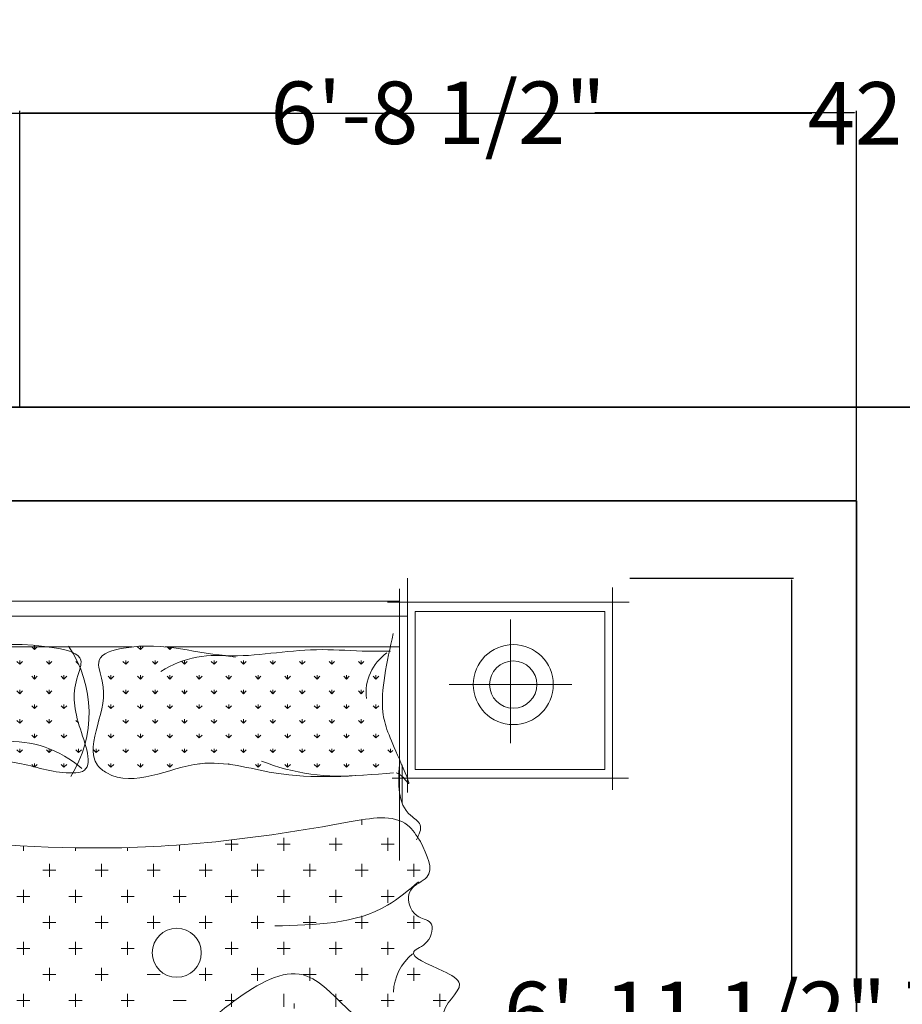
# Model space of a CAD drawing. Units: inches. Extents: x -26 to 575, y -18 to 513.
# Tile 14 of 28: x 189 to 274, y 418 to 513. Entities that reach past the tile are written whole.
import ezdxf

# ---------------------------------------------------------------- set-up
doc = ezdxf.new("R2010")
doc.units = ezdxf.units.IN
doc.header["$MEASUREMENT"] = 0
for name, color, linetype, lineweight in [('A-ANNO-DIMS', 2, 'Continuous', 18), ('A-WALL', 7, 'Continuous', 35), ('Furniture', 8, 'Continuous', 15)]:
    doc.layers.add(name, color=color, linetype=linetype, lineweight=lineweight)
doc.styles.get("Standard").update_dxf_attribs({"font": 'arial.ttf', "height": 6})
doc.dimstyles.get("Standard").update_dxf_attribs({"dimtxt": 6, "dimasz": 0.18, "dimexe": 0.18, "dimexo": 0.0625, "dimgap": 0.09, "dimtad": 0, "dimtih": 1, "dimtoh": 1, "dimzin": 0, "dimdsep": 46, "dimlunit": 3, "dimtxsty": 'Standard', "dimcen": 0.09, "dimadec": 0, "dimazin": 0, "dimtfac": 1, "dimtofl": 0, "dimtmove": 0, "dimatfit": 3, "dimfxl": 1, "dimtolj": 1, "dimtzin": 0, "dimarcsym": 0})

# ---------------------------------------------------------------- blocks, each defined once
blk = doc.blocks.new('*D1')
at = {"layer": 'A-ANNO-DIMS', "color": 0, "lineweight": -2, "transparency": 16777216}
for p, q in [((18.177, 475.57), (18.177, 503.937)), ((18.357, 503.757), (264.875, 503.757)), ((521.997, 503.757), (275.479, 503.757)), ((522.177, 475.57), (522.177, 503.937))]:
    blk.add_line(p, q, dxfattribs=at)
at = {"layer": 'A-ANNO-DIMS', "color": 0, "transparency": 16777216}
for points in [[(18.357, 503.787), (18.357, 503.727), (18.177, 503.757)], [(521.997, 503.787), (521.997, 503.727), (522.177, 503.757)]]:
    blk.add_solid(points, dxfattribs=at)
at = {"layer": 'Defpoints', "color": 0, "transparency": 16777216}
for p in [(522.177, 503.757), (18.177, 475.508), (522.177, 475.508)]:
    blk.add_point(p, dxfattribs=at)
at = {"layer": 'A-ANNO-DIMS', "color": 0, "transparency": 16777216, "insert": (270.177, 503.757), "char_height": 6, "attachment_point": 5}
blk.add_mtext("\\A1;42'", dxfattribs=at)
blk = doc.blocks.new('BED-DOUBLE-WITH-NIGHTSTANDS')
for p, q in [((82.669, 83.361), (82.669, 62.761)), ((81.883, 82.344), (81.883, 56.232)), ((102.354, 63.031), (102.354, 82.461)), ((21.24, 81.17), (81.883, 81.17)), ((103.97, 81.078), (80.744, 81.078)), ((82.669, 79.717), (21.062, 79.717)), ((101.633, 80.153), (83.411, 80.153)), ((83.411, 80.153), (83.411, 64.968)), ((101.633, 64.968), (101.633, 80.153)), ((92.567, 79.403), (92.567, 67.508)), ((56.226, 76.764), (41.357, 76.764)), ((46.825, 76.507), (46.56, 76.772)), ((46.825, 76.507), (47.09, 76.772)), ((46.826, 76.507), (46.826, 76.882)), ((57.003, 76.507), (56.737, 76.772)), ((57.003, 76.507), (57.003, 76.828)), ((57.003, 76.507), (57.268, 76.772)), ((81.883, 76.764), (59.394, 76.764)), ((59.831, 76.507), (59.594, 76.744)), ((59.831, 76.507), (59.831, 76.717)), ((59.831, 76.507), (60.018, 76.694)), ((45.411, 75.093), (45.146, 75.358)), ((45.411, 75.093), (45.411, 75.468)), ((45.411, 75.093), (45.676, 75.358)), ((48.239, 75.093), (47.974, 75.358)), ((48.239, 75.093), (48.505, 75.358)), ((48.24, 75.093), (48.24, 75.468)), ((51.068, 75.093), (50.803, 75.358)), ((51.068, 75.093), (51.068, 75.099)), ((51.068, 75.093), (51.07, 75.095)), ((53.004, 75.337), (53.025, 75.358)), ((55.588, 75.093), (55.323, 75.358)), ((55.588, 75.093), (55.854, 75.358)), ((55.589, 75.093), (55.589, 75.468)), ((58.417, 75.093), (58.152, 75.358)), ((58.417, 75.093), (58.417, 75.468)), ((58.417, 75.093), (58.682, 75.358)), ((61.245, 75.093), (60.98, 75.358)), ((61.245, 75.093), (61.51, 75.358)), ((61.246, 75.093), (61.246, 75.468)), ((64.074, 75.093), (63.809, 75.358)), ((64.074, 75.093), (64.074, 75.468)), ((64.074, 75.093), (64.339, 75.358)), ((66.902, 75.093), (66.637, 75.358)), ((66.902, 75.093), (67.167, 75.358)), ((66.903, 75.093), (66.903, 75.468)), ((69.731, 75.093), (69.465, 75.358)), ((69.731, 75.093), (69.731, 75.468)), ((69.731, 75.093), (69.996, 75.358)), ((72.559, 75.093), (72.294, 75.358)), ((72.559, 75.093), (72.559, 75.468)), ((72.559, 75.093), (72.824, 75.358)), ((75.387, 75.093), (75.122, 75.358)), ((75.387, 75.093), (75.653, 75.358)), ((75.388, 75.093), (75.388, 75.468)), ((78.216, 75.093), (77.951, 75.358)), ((78.216, 75.093), (78.216, 75.468)), ((78.216, 75.093), (78.481, 75.358)), ((46.825, 73.679), (46.56, 73.944)), ((46.825, 73.679), (47.09, 73.944)), ((46.826, 73.678), (46.826, 74.053)), ((49.654, 73.679), (49.388, 73.944)), ((49.654, 73.678), (49.654, 74.053)), ((49.654, 73.679), (49.919, 73.944)), ((54.174, 73.679), (53.909, 73.944)), ((54.174, 73.679), (54.439, 73.944)), ((54.175, 73.678), (54.175, 74.053)), ((57.003, 73.679), (56.737, 73.944)), ((57.003, 73.678), (57.003, 74.053)), ((57.003, 73.679), (57.268, 73.944)), ((59.831, 73.679), (59.566, 73.944)), ((59.831, 73.678), (59.831, 74.053)), ((59.831, 73.679), (60.096, 73.944)), ((62.66, 73.679), (62.394, 73.944)), ((62.66, 73.678), (62.66, 74.053)), ((62.66, 73.679), (62.925, 73.944)), ((65.488, 73.679), (65.223, 73.944)), ((65.488, 73.678), (65.488, 74.053)), ((65.488, 73.679), (65.753, 73.944)), ((68.316, 73.679), (68.051, 73.944)), ((68.316, 73.679), (68.582, 73.944)), ((68.317, 73.678), (68.317, 74.053)), ((71.145, 73.679), (70.88, 73.944)), ((71.145, 73.678), (71.145, 74.053)), ((71.145, 73.679), (71.41, 73.944)), ((73.973, 73.679), (73.708, 73.944)), ((73.973, 73.679), (74.238, 73.944)), ((73.974, 73.678), (73.974, 74.053)), ((76.802, 73.679), (76.536, 73.944)), ((76.802, 73.678), (76.802, 74.053)), ((76.802, 73.679), (77.067, 73.944)), ((79.63, 73.679), (79.365, 73.944)), ((79.63, 73.678), (79.63, 74.053)), ((79.63, 73.679), (79.895, 73.944)), ((98.466, 73.144), (86.668, 73.144)), ((45.411, 72.265), (45.146, 72.53)), ((45.411, 72.264), (45.411, 72.639)), ((45.411, 72.265), (45.676, 72.53)), ((48.239, 72.265), (47.974, 72.53)), ((48.239, 72.265), (48.505, 72.53)), ((48.24, 72.264), (48.24, 72.639)), ((55.588, 72.265), (55.323, 72.53)), ((55.588, 72.265), (55.854, 72.53)), ((55.589, 72.264), (55.589, 72.639)), ((58.417, 72.265), (58.152, 72.53)), ((58.417, 72.264), (58.417, 72.639)), ((58.417, 72.265), (58.682, 72.53)), ((61.245, 72.265), (60.98, 72.53)), ((61.245, 72.265), (61.51, 72.53)), ((61.246, 72.264), (61.246, 72.639)), ((64.074, 72.265), (63.809, 72.53)), ((64.074, 72.264), (64.074, 72.639)), ((64.074, 72.265), (64.339, 72.53)), ((66.902, 72.265), (66.637, 72.53)), ((66.902, 72.265), (67.167, 72.53)), ((66.903, 72.264), (66.903, 72.639)), ((69.731, 72.265), (69.465, 72.53)), ((69.731, 72.264), (69.731, 72.639)), ((69.731, 72.265), (69.996, 72.53)), ((72.559, 72.265), (72.294, 72.53)), ((72.559, 72.264), (72.559, 72.639)), ((72.559, 72.265), (72.824, 72.53)), ((75.387, 72.265), (75.122, 72.53)), ((75.387, 72.265), (75.653, 72.53)), ((75.388, 72.264), (75.388, 72.639)), ((78.216, 72.265), (77.951, 72.53)), ((78.216, 72.264), (78.216, 72.639)), ((78.216, 72.265), (78.481, 72.53)), ((46.825, 70.85), (46.56, 71.116)), ((46.825, 70.85), (47.09, 71.116)), ((46.826, 70.85), (46.826, 71.225)), ((49.654, 70.85), (49.388, 71.116)), ((49.654, 70.85), (49.654, 71.225)), ((49.654, 70.85), (49.919, 71.116)), ((54.174, 70.85), (53.909, 71.116)), ((54.174, 70.85), (54.439, 71.116)), ((54.175, 70.85), (54.175, 71.225)), ((57.003, 70.85), (56.737, 71.116)), ((57.003, 70.85), (57.003, 71.225)), ((57.003, 70.85), (57.268, 71.116)), ((59.831, 70.85), (59.566, 71.116)), ((59.831, 70.85), (59.831, 71.225)), ((59.831, 70.85), (60.096, 71.116)), ((62.66, 70.85), (62.394, 71.116)), ((62.66, 70.85), (62.66, 71.225)), ((62.66, 70.85), (62.925, 71.116)), ((65.488, 70.85), (65.223, 71.116)), ((65.488, 70.85), (65.488, 71.225)), ((65.488, 70.85), (65.753, 71.116)), ((68.316, 70.85), (68.051, 71.116)), ((68.316, 70.85), (68.582, 71.116)), ((68.317, 70.85), (68.317, 71.225)), ((71.145, 70.85), (70.88, 71.116)), ((71.145, 70.85), (71.145, 71.225)), ((71.145, 70.85), (71.41, 71.116)), ((73.973, 70.85), (73.708, 71.116)), ((73.973, 70.85), (74.238, 71.116)), ((73.974, 70.85), (73.974, 71.225)), ((76.802, 70.85), (76.536, 71.116)), ((76.802, 70.85), (76.802, 71.225)), ((76.802, 70.85), (77.067, 71.116)), ((79.63, 70.85), (79.365, 71.116)), ((79.63, 70.85), (79.63, 71.225)), ((79.63, 70.85), (79.895, 71.116)), ((45.411, 69.436), (45.146, 69.701)), ((45.411, 69.436), (45.411, 69.811)), ((45.411, 69.436), (45.676, 69.701)), ((48.239, 69.436), (47.974, 69.701)), ((48.239, 69.436), (48.505, 69.701)), ((48.24, 69.436), (48.24, 69.811)), ((51.052, 69.452), (50.803, 69.701)), ((53.007, 69.683), (53.025, 69.701)), ((55.588, 69.436), (55.323, 69.701)), ((55.588, 69.436), (55.854, 69.701)), ((55.589, 69.436), (55.589, 69.811)), ((58.417, 69.436), (58.152, 69.701)), ((58.417, 69.436), (58.417, 69.811)), ((58.417, 69.436), (58.682, 69.701)), ((61.245, 69.436), (60.98, 69.701)), ((61.245, 69.436), (61.51, 69.701)), ((61.246, 69.436), (61.246, 69.811)), ((64.074, 69.436), (63.809, 69.701)), ((64.074, 69.436), (64.074, 69.811)), ((64.074, 69.436), (64.339, 69.701)), ((66.902, 69.436), (66.637, 69.701)), ((66.902, 69.436), (67.167, 69.701)), ((66.903, 69.436), (66.903, 69.811)), ((69.731, 69.436), (69.465, 69.701)), ((69.731, 69.436), (69.731, 69.811)), ((69.731, 69.436), (69.996, 69.701)), ((72.559, 69.436), (72.294, 69.701)), ((72.559, 69.436), (72.559, 69.811)), ((72.559, 69.436), (72.824, 69.701)), ((75.387, 69.436), (75.122, 69.701)), ((75.387, 69.436), (75.653, 69.701)), ((75.388, 69.436), (75.388, 69.811)), ((78.216, 69.436), (77.951, 69.701)), ((78.216, 69.436), (78.216, 69.811)), ((78.216, 69.436), (78.481, 69.701)), ((46.825, 68.022), (46.56, 68.287)), ((46.825, 68.022), (47.09, 68.287)), ((46.826, 68.022), (46.826, 68.397)), ((49.654, 68.022), (49.388, 68.287)), ((49.654, 68.022), (49.654, 68.397)), ((49.654, 68.022), (49.919, 68.287)), ((54.174, 68.022), (53.909, 68.287)), ((54.174, 68.022), (54.439, 68.287)), ((54.175, 68.022), (54.175, 68.397)), ((57.003, 68.022), (56.737, 68.287)), ((57.003, 68.022), (57.003, 68.397)), ((57.003, 68.022), (57.268, 68.287)), ((59.831, 68.022), (59.566, 68.287)), ((59.831, 68.022), (59.831, 68.397)), ((59.831, 68.022), (60.096, 68.287)), ((62.66, 68.022), (62.394, 68.287)), ((62.66, 68.022), (62.66, 68.397)), ((62.66, 68.022), (62.925, 68.287)), ((65.488, 68.022), (65.223, 68.287)), ((65.488, 68.022), (65.488, 68.397)), ((65.488, 68.022), (65.753, 68.287)), ((68.316, 68.022), (68.051, 68.287)), ((68.316, 68.022), (68.582, 68.287)), ((68.317, 68.022), (68.317, 68.397)), ((71.145, 68.022), (70.88, 68.287)), ((71.145, 68.022), (71.145, 68.397)), ((71.145, 68.022), (71.41, 68.287)), ((73.973, 68.022), (73.708, 68.287)), ((73.973, 68.022), (74.238, 68.287)), ((73.974, 68.022), (73.974, 68.397)), ((76.802, 68.022), (76.536, 68.287)), ((76.802, 68.022), (76.802, 68.397)), ((76.802, 68.022), (77.067, 68.287)), ((79.63, 68.022), (79.365, 68.287)), ((79.63, 68.022), (79.63, 68.397)), ((79.63, 68.022), (79.895, 68.287)), ((45.411, 66.608), (45.146, 66.873)), ((45.411, 66.607), (45.411, 66.982)), ((45.411, 66.608), (45.676, 66.873)), ((48.239, 66.608), (47.974, 66.873)), ((48.239, 66.608), (48.505, 66.873)), ((48.24, 66.607), (48.24, 66.982)), ((51.068, 66.608), (50.803, 66.873)), ((51.068, 66.607), (51.068, 66.982)), ((51.068, 66.608), (51.333, 66.873)), ((52.76, 66.608), (52.495, 66.873)), ((52.76, 66.607), (52.76, 66.982)), ((52.76, 66.608), (53.025, 66.873)), ((55.588, 66.608), (55.323, 66.873)), ((55.588, 66.608), (55.854, 66.873)), ((55.589, 66.607), (55.589, 66.982)), ((58.417, 66.608), (58.152, 66.873)), ((58.417, 66.607), (58.417, 66.982)), ((58.417, 66.608), (58.682, 66.873)), ((61.245, 66.608), (60.98, 66.873)), ((61.245, 66.608), (61.51, 66.873)), ((61.246, 66.607), (61.246, 66.982)), ((64.074, 66.608), (63.809, 66.873)), ((64.074, 66.607), (64.074, 66.982)), ((64.074, 66.608), (64.339, 66.873)), ((66.902, 66.608), (66.637, 66.873)), ((66.902, 66.608), (67.167, 66.873)), ((66.903, 66.607), (66.903, 66.982)), ((69.731, 66.608), (69.465, 66.873)), ((69.731, 66.607), (69.731, 66.982)), ((69.731, 66.608), (69.996, 66.873)), ((72.559, 66.608), (72.294, 66.873)), ((72.559, 66.607), (72.559, 66.982)), ((72.559, 66.608), (72.824, 66.873)), ((75.387, 66.608), (75.122, 66.873)), ((75.387, 66.608), (75.653, 66.873)), ((75.388, 66.607), (75.388, 66.982)), ((78.216, 66.608), (77.951, 66.873)), ((78.216, 66.607), (78.216, 66.982)), ((78.216, 66.608), (78.481, 66.873)), ((81.044, 66.608), (80.779, 66.873)), ((81.044, 66.608), (81.253, 66.817)), ((81.045, 66.607), (81.045, 66.982)), ((46.774, 65.245), (46.56, 65.459)), ((46.826, 65.232), (46.826, 65.568)), ((46.856, 65.224), (47.09, 65.459)), ((49.654, 65.194), (49.388, 65.459)), ((49.654, 65.193), (49.654, 65.568)), ((49.654, 65.194), (49.919, 65.459)), ((54.174, 65.194), (53.909, 65.459)), ((54.174, 65.194), (54.439, 65.459)), ((54.175, 65.193), (54.175, 65.568)), ((57.003, 65.194), (56.737, 65.459)), ((57.003, 65.193), (57.003, 65.568)), ((57.003, 65.194), (57.268, 65.459)), ((59.831, 65.194), (59.566, 65.459)), ((59.831, 65.193), (59.831, 65.568)), ((59.831, 65.194), (60.096, 65.459)), ((62.66, 65.525), (62.66, 65.568)), ((65.488, 65.481), (65.488, 65.568)), ((65.74, 65.446), (65.753, 65.459)), ((68.316, 65.194), (68.051, 65.459)), ((68.316, 65.194), (68.582, 65.459)), ((68.317, 65.193), (68.317, 65.568)), ((71.145, 65.194), (70.88, 65.459)), ((71.145, 65.193), (71.145, 65.568)), ((71.145, 65.194), (71.41, 65.459)), ((73.973, 65.194), (73.708, 65.459)), ((73.973, 65.194), (74.238, 65.459)), ((73.974, 65.193), (73.974, 65.568)), ((76.802, 65.194), (76.536, 65.459)), ((76.802, 65.193), (76.802, 65.568)), ((76.802, 65.194), (77.067, 65.459)), ((79.63, 65.194), (79.365, 65.459)), ((79.63, 65.193), (79.63, 65.568)), ((79.63, 65.194), (79.895, 65.459)), ((82.154, 61.735), (82.154, 65.422)), ((83.411, 64.968), (101.633, 64.968)), ((55.589, 64.121), (55.589, 64.154)), ((81.194, 64.149), (103.88, 64.149)), ((78.267, 59.667), (78.267, 60.149)), ((60.767, 57.167), (60.767, 57.735)), ((66.392, 57.792), (65.142, 57.792)), ((65.767, 57.167), (65.767, 58.213)), ((71.392, 57.792), (70.142, 57.792)), ((70.767, 57.167), (70.767, 58.417)), ((76.392, 57.792), (75.142, 57.792)), ((75.767, 57.167), (75.767, 58.417)), ((81.392, 57.792), (80.142, 57.792)), ((80.767, 57.167), (80.767, 58.417)), ((45.767, 57.167), (45.767, 57.639)), ((50.767, 57.167), (50.767, 57.462)), ((55.767, 57.167), (55.767, 57.483)), ((48.267, 54.667), (48.267, 55.917)), ((53.267, 54.667), (53.267, 55.917)), ((58.267, 54.667), (58.267, 55.917)), ((63.267, 54.667), (63.267, 55.917)), ((68.267, 54.667), (68.267, 55.917)), ((73.267, 54.667), (73.267, 55.917)), ((78.267, 54.667), (78.267, 55.917)), ((83.267, 54.667), (83.267, 55.917)), ((48.892, 55.292), (47.642, 55.292)), ((53.892, 55.292), (52.642, 55.292)), ((58.892, 55.292), (57.642, 55.292)), ((63.892, 55.292), (62.642, 55.292)), ((68.892, 55.292), (67.642, 55.292)), ((73.892, 55.292), (72.642, 55.292)), ((78.892, 55.292), (77.642, 55.292)), ((83.892, 55.292), (82.642, 55.292)), ((45.767, 52.167), (45.767, 53.417)), ((50.767, 52.167), (50.767, 53.417)), ((55.767, 52.167), (55.767, 53.417)), ((60.767, 52.167), (60.767, 53.417)), ((65.767, 52.167), (65.767, 53.417)), ((70.767, 52.167), (70.767, 53.417)), ((75.767, 52.167), (75.767, 53.417)), ((80.767, 52.167), (80.767, 53.417)), ((46.392, 52.792), (45.142, 52.792)), ((51.392, 52.792), (50.142, 52.792)), ((56.392, 52.792), (55.142, 52.792)), ((61.392, 52.792), (60.142, 52.792)), ((66.392, 52.792), (65.142, 52.792)), ((71.392, 52.792), (70.142, 52.792)), ((76.392, 52.792), (75.142, 52.792)), ((81.392, 52.792), (80.142, 52.792)), ((48.892, 50.292), (47.642, 50.292)), ((48.267, 49.667), (48.267, 50.917)), ((53.892, 50.292), (52.642, 50.292)), ((53.267, 49.667), (53.267, 50.917)), ((58.892, 50.292), (57.642, 50.292)), ((58.267, 49.667), (58.267, 50.917)), ((63.892, 50.292), (62.642, 50.292)), ((63.267, 49.667), (63.267, 50.917)), ((68.892, 50.292), (67.642, 50.292)), ((68.267, 49.667), (68.267, 50.917)), ((73.892, 50.292), (72.642, 50.292)), ((73.267, 49.667), (73.267, 50.917)), ((78.892, 50.292), (77.642, 50.292)), ((78.267, 49.667), (78.267, 50.917)), ((83.892, 50.292), (82.642, 50.292)), ((83.267, 49.667), (83.267, 50.917)), ((45.767, 47.167), (45.767, 48.417)), ((50.767, 47.167), (50.767, 48.417)), ((55.767, 47.167), (55.767, 48.417)), ((65.767, 47.167), (65.767, 48.417)), ((70.767, 47.167), (70.767, 48.417)), ((75.767, 47.167), (75.767, 48.417)), ((80.767, 47.167), (80.767, 48.417)), ((46.392, 47.792), (45.142, 47.792)), ((51.392, 47.792), (50.142, 47.792)), ((56.392, 47.792), (55.142, 47.792)), ((66.392, 47.792), (65.142, 47.792)), ((71.392, 47.792), (70.142, 47.792)), ((76.392, 47.792), (75.142, 47.792)), ((81.392, 47.792), (80.142, 47.792)), ((48.267, 44.667), (48.267, 45.917)), ((53.267, 44.667), (53.267, 45.917)), ((63.267, 44.667), (63.267, 45.917)), ((68.267, 44.667), (68.267, 45.917)), ((73.267, 44.667), (73.267, 45.917)), ((78.267, 44.667), (78.267, 45.917)), ((83.267, 44.667), (83.267, 45.917)), ((48.892, 45.292), (47.642, 45.292)), ((53.892, 45.292), (52.642, 45.292)), ((58.892, 45.292), (57.642, 45.292)), ((63.892, 45.292), (62.642, 45.292)), ((68.892, 45.292), (67.642, 45.292)), ((73.892, 45.292), (72.642, 45.292)), ((78.892, 45.292), (77.642, 45.292)), ((83.892, 45.292), (82.642, 45.292)), ((46.392, 42.792), (45.142, 42.792)), ((45.767, 42.167), (45.767, 43.417)), ((51.392, 42.792), (50.142, 42.792)), ((50.767, 42.167), (50.767, 43.417)), ((56.392, 42.792), (55.142, 42.792)), ((55.767, 42.167), (55.767, 43.417)), ((61.392, 42.792), (60.142, 42.792)), ((66.089, 42.792), (65.142, 42.792)), ((65.767, 42.167), (65.767, 43.417)), ((70.767, 42.167), (70.767, 43.417)), ((75.767, 42.167), (75.767, 43.417)), ((76.392, 42.792), (76.07, 42.792)), ((81.392, 42.792), (80.142, 42.792)), ((80.767, 42.167), (80.767, 43.417)), ((86.392, 42.792), (85.142, 42.792)), ((85.767, 42.167), (85.767, 43.417)), ((71.779, 42.017), (71.779, 42.495))]:
    blk.add_line(p, q)
for centre, radius in [((92.824, 73.144), 3.847), ((92.824, 73.144), 2.272), ((60.492, 47.373), 2.359)]:
    blk.add_circle(centre, radius)
for centre, radius, start, end in [((40.615, 70.411), 11.457, 327.75554, 34.13971), ((64.238, 66.161), 9.788, 78.78839, 122.5362), ((83.338, 72.35), 4.658, 124.73446, 186.55264), ((44.415, 57.102), 10.589, 48.87132, 93.34478), ((76.199, 84.696), 20.356, 248.18569, 275.91055), ((86.259, 43.416), 4.944, 128.83543, 178.00379)]:
    blk.add_arc(centre, radius, start, end)
for points, knots in [([(24.713, 64.661), (26.06, 64.632), (33.003, 64.48), (41.955, 67.204), (49.025, 64.485), (52.786, 64.865), (50.633, 69.88), (50.431, 72.758), (51.756, 76.03), (43.447, 78.051), (36.588, 75.072), (28.311, 76.389), (25.374, 76.358), (24.839, 76.353)], [0, 0, 0, 0, 4.049674, 20.880819, 25.932041, 26.821979, 31.217024, 36.043065, 37.533831, 40.150607, 55.448466, 62.672935, 64.278467, 64.278467, 64.278467, 64.278467]), ([(81.301, 78.042), (80.682, 75.308), (79.671, 70.849), (81.18, 67.616), (83.379, 62.518), (82.094, 64.567), (81.589, 64.661)], [0, 0, 0, 0, 7.603099, 12.404488, 14.892294, 16.432626, 16.432626, 16.432626, 16.432626]), ([(81.33, 64.661), (77.466, 64.343), (71.206, 63.827), (62.265, 66.782), (55.978, 62.892), (52.048, 65.922), (52.93, 69.57), (53.856, 72.566), (52.444, 75.929), (58.704, 77.688), (63.648, 75.449), (70.131, 76.236), (74.451, 76.625), (78.12, 76.323), (80.316, 76.345), (81.042, 76.353)], [0, 0, 0, 0, 11.502554, 18.635017, 27.654655, 28.800011, 32.595859, 36.914018, 38.927328, 41.544104, 52.009639, 56.262652, 60.661637, 65.075538, 67.252844, 67.252844, 67.252844, 67.252844]), ([(81.883, 65.422), (81.768, 63.582), (81.624, 61.268), (84.254, 59.709), (83.774, 58.738), (83.516, 58.215)], [0, 0, 0, 0, 4.973031, 6.254082, 7.747585, 7.747585, 7.747585, 7.747585]), ([(83.91, 58.069), (84.557, 56.735), (85.575, 54.637), (82.278, 53.65), (82.991, 50.721), (85.334, 50.529), (84.903, 48.234), (82.063, 47.247), (85.774, 45.875), (88.761, 44.174), (85.372, 42.034), (87.053, 39.3), (78.856, 37.339), (72.977, 51.01), (54.082, 29.239), (35.907, 32.924), (20.82, 41.987), (17.166, 32.566), (16.239, 37.799), (18.713, 38.787), (15.912, 43.442), (22.37, 43.447), (20.934, 46.182), (20.192, 47.949), (20.317, 52.932), (35.125, 52.602), (16.252, 58.944), (26.308, 59.478), (35.165, 58.384), (54.321, 56.67), (69.444, 58.458), (82.072, 60.876), (83.528, 58.651), (83.91, 58.069)], [0, 0, 0, 0, 3.481099, 5.475811, 8.043407, 9.436812, 11.330727, 12.888379, 16.258255, 18.252967, 21.734596, 23.018392, 26.087149, 38.445812, 54.5649, 86.600283, 92.594507, 98.286547, 100.905288, 101.70342, 105.471876, 109.954916, 110.954151, 113.598333, 116.114301, 124.231953, 133.25029, 137.509046, 143.991555, 164.906349, 189.961005, 195.579007, 197.573325, 197.573325, 197.573325, 197.573325]), ([(83.725, 54.2), (82.764, 53.378), (78.971, 50.136), (73.792, 50.033), (69.926, 49.956)], [0, 0, 0, 0, 3.737027, 14.742384, 14.742384, 14.742384, 14.742384])]:
    blk.add_open_spline(points, degree=3, knots=knots)
blk = doc.blocks.new('*D13')
at = {"layer": 'A-ANNO-DIMS', "color": 0, "lineweight": -2, "transparency": 16777216}
for p, q in [((247.41, 459.077), (263.123, 459.077)), ((262.943, 458.897), (262.943, 420.496)), ((262.943, 375.711), (262.943, 414.111)), ((247.41, 375.531), (263.123, 375.531))]:
    blk.add_line(p, q, dxfattribs=at)
at = {"layer": 'A-ANNO-DIMS', "color": 0, "transparency": 16777216}
for points in [[(262.913, 458.897), (262.973, 458.897), (262.943, 459.077)], [(262.913, 375.711), (262.973, 375.711), (262.943, 375.531)]]:
    blk.add_solid(points, dxfattribs=at)
at = {"layer": 'Defpoints', "color": 0, "transparency": 16777216}
for p in [(247.348, 459.077), (262.943, 459.077), (247.348, 375.531)]:
    blk.add_point(p, dxfattribs=at)
at = {"layer": 'A-ANNO-DIMS', "color": 0, "transparency": 16777216, "insert": (262.943, 417.304), "char_height": 6, "attachment_point": 5}
blk.add_mtext('\\A1;6\'-11 1/2" TYP.', dxfattribs=at)
blk = doc.blocks.new('*D30')
at = {"layer": 'A-ANNO-DIMS', "color": 0, "lineweight": -2, "transparency": 16777216}
for p, q in [((188.784, 475.57), (188.784, 503.988)), ((188.964, 503.808), (213.909, 503.808)), ((268.997, 503.808), (244.052, 503.808)), ((269.177, 466.57), (269.177, 503.988))]:
    blk.add_line(p, q, dxfattribs=at)
at = {"layer": 'A-ANNO-DIMS', "color": 0, "transparency": 16777216}
for points in [[(188.964, 503.838), (188.964, 503.778), (188.784, 503.808)], [(268.997, 503.838), (268.997, 503.778), (269.177, 503.808)]]:
    blk.add_solid(points, dxfattribs=at)
at = {"layer": 'Defpoints', "color": 0, "transparency": 16777216}
for p in [(269.177, 503.808), (188.784, 475.508), (269.177, 466.508)]:
    blk.add_point(p, dxfattribs=at)
at = {"layer": 'A-ANNO-DIMS', "color": 0, "transparency": 16777216, "insert": (228.981, 503.808), "char_height": 6, "attachment_point": 5}
blk.add_mtext('\\A1;6\'-8 1/2"', dxfattribs=at)

msp = doc.modelspace()

# ---------------------------------------------------------------- linework, layer by layer
at = {"layer": 'A-WALL'}
for p, q in [((269.177, 466.508), (138.677, 466.508)), ((269.177, 334.508), (269.177, 466.508))]:
    msp.add_line(p, q, dxfattribs=at)
msp.add_lwpolyline([(18.177, 19.508), (522.177, 19.508), (522.177, 475.508), (18.177, 475.508)], close=True, dxfattribs=at)

# ---------------------------------------------------------------- block references
at = {"layer": 'Furniture'}
msp.add_blockref('BED-DOUBLE-WITH-NIGHTSTANDS', (143.378, 375.716), dxfattribs=at)

# ---------------------------------------------------------------- dimensions: what is measured, and where the dimension line sits
at = {"layer": 'A-ANNO-DIMS'}
for base, p1, p2, override, picture, middle in [((269.177, 503.808), (188.784, 475.508), (269.177, 466.508), {"dimdec": 1, "dimlfac": 1, "dimrnd": 0, "dimzin": 1, "dimdsep": 46, "dimlunit": 4, "dimfrac": 2}, '*D30', (228.981, 503.808)), ((522.177, 503.757), (18.177, 475.508), (522.177, 475.508), {"dimclrd": 0, "dimclre": 0, "dimclrt": 0}, '*D1', (270.177, 503.757))]:
    dim = msp.add_linear_dim(base=base, p1=p1, p2=p2, dimstyle='Standard', override=override, dxfattribs=at)
    dim.commit()
    dim.dimension.update_dxf_attribs({"geometry": picture, "text_midpoint": middle})
dim = msp.add_linear_dim(base=(262.943, 459.077), p1=(247.348, 375.531), p2=(247.348, 459.077), angle=90, text='<> TYP.', dimstyle='Standard', override={"dimdec": 1, "dimlfac": 1, "dimrnd": 0, "dimzin": 1, "dimdsep": 46, "dimlunit": 4, "dimfrac": 2}, dxfattribs=at)
dim.commit()
dim.dimension.update_dxf_attribs({"geometry": '*D13', "text_midpoint": (262.943, 417.304)})

doc.saveas('drawing.dxf')
